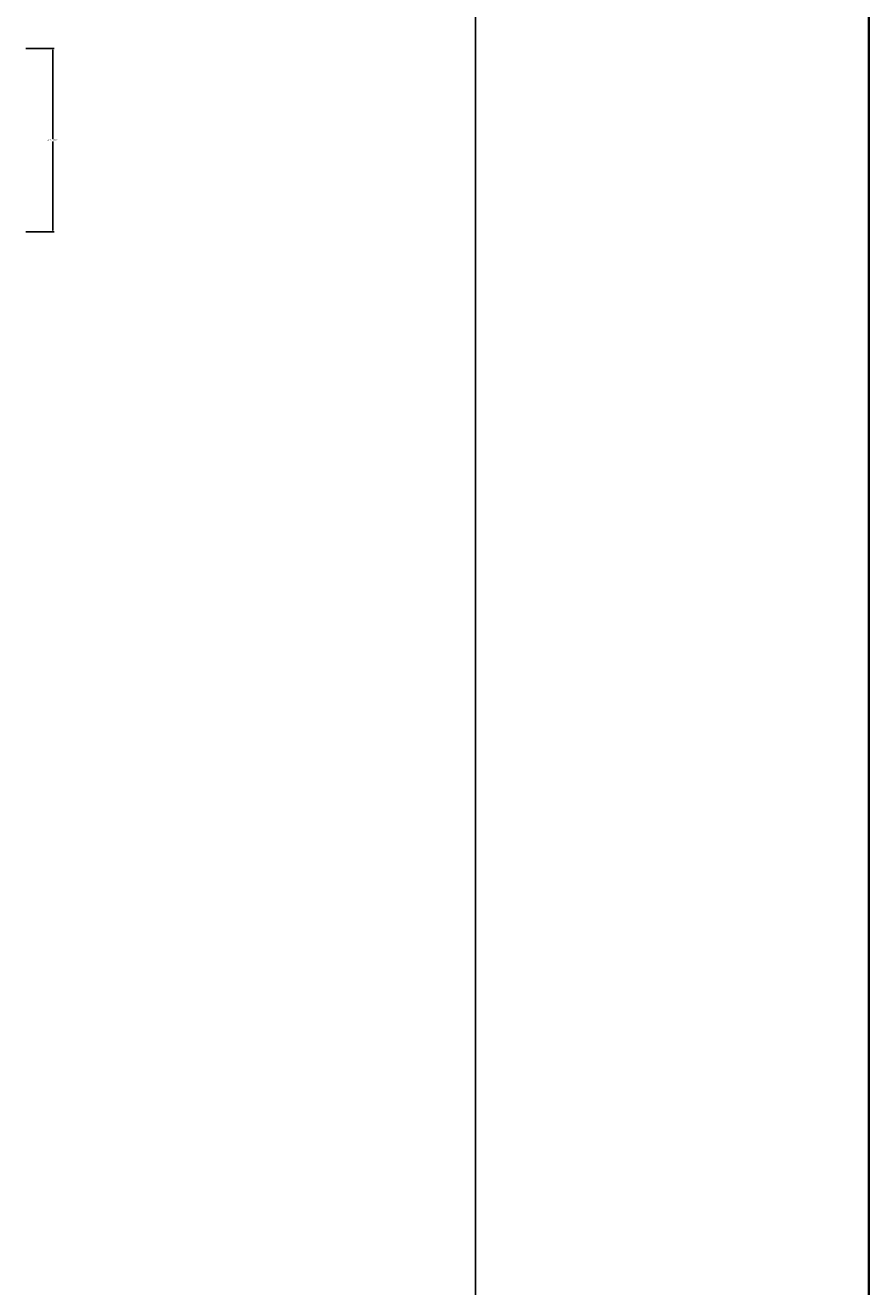
# Model space of a CAD drawing. Units: inches. Extents: x 1962 to 2771, y 1245 to 2660.
# Tile 19 of 114: x 2661 to 2771, y 1527 to 1692. Entities that reach past the tile are written whole.
import ezdxf

# ---------------------------------------------------------------- set-up
doc = ezdxf.new("R2010")
doc.units = ezdxf.units.IN
doc.layers.add('A-ANNO-DIMS', color=2, linetype='Continuous', lineweight=18)
doc.layers.add('A-ANNO-TTLB', color=7, linetype='Continuous', lineweight=35)
doc.styles.get("Standard").update_dxf_attribs({"font": 'arial.ttf'})
doc.dimstyles.get("Standard").update_dxf_attribs({"dimtxt": 0.18, "dimasz": 0.18, "dimexe": 0.18, "dimexo": 0.0625, "dimgap": 0.09, "dimtad": 0, "dimtih": 1, "dimtoh": 1, "dimdec": 4, "dimzin": 0, "dimdsep": 46, "dimtxsty": 'Standard', "dimcen": 0.09, "dimadec": 0, "dimazin": 0, "dimtfac": 1, "dimtdec": 4, "dimtofl": 0, "dimtmove": 0, "dimatfit": 3, "dimfxl": 1, "dimtolj": 1, "dimtzin": 0, "dimarcsym": 0})

# ---------------------------------------------------------------- blocks, each defined once
blk = doc.blocks.new('*D18')
at = {"layer": 'A-ANNO-DIMS', "color": 0, "lineweight": -2, "transparency": 16777216}
for p, q in [((2660.87, 1688.97), (2664.59, 1688.97)), ((2664.41, 1688.79), (2664.41, 1677.15)), ((2664.41, 1665.15), (2664.41, 1676.79)), ((2660.87, 1664.97), (2664.59, 1664.97))]:
    blk.add_line(p, q, dxfattribs=at)
at = {"layer": 'A-ANNO-DIMS', "color": 0, "transparency": 16777216}
for points in [[(2664.38, 1688.79), (2664.44, 1688.79), (2664.41, 1688.97)], [(2664.38, 1665.15), (2664.44, 1665.15), (2664.41, 1664.97)]]:
    blk.add_solid(points, dxfattribs=at)
at = {"layer": 'Defpoints', "color": 0, "transparency": 16777216}
for p in [(2660.81, 1688.97), (2664.41, 1688.97), (2660.81, 1664.97)]:
    blk.add_point(p, dxfattribs=at)
at = {"layer": 'A-ANNO-DIMS', "color": 0, "transparency": 16777216, "insert": (2664.41, 1676.97), "char_height": 0.18, "attachment_point": 5}
blk.add_mtext('\\A1;W1A 24 TYP.', dxfattribs=at)
blk = doc.blocks.new('*D42')
at = {"layer": 'A-ANNO-DIMS', "color": 0, "lineweight": -2, "transparency": 16777216}
for p, q in [((2660.87, 2524.34), (2719.94, 2524.34)), ((2719.76, 2524.16), (2719.76, 1979.28)), ((2719.76, 1434.02), (2719.76, 1978.91)), ((2660.87, 1433.84), (2719.94, 1433.84))]:
    blk.add_line(p, q, dxfattribs=at)
at = {"layer": 'A-ANNO-DIMS', "color": 0, "transparency": 16777216}
for points in [[(2719.73, 2524.16), (2719.79, 2524.16), (2719.76, 2524.34)], [(2719.73, 1434.02), (2719.79, 1434.02), (2719.76, 1433.84)]]:
    blk.add_solid(points, dxfattribs=at)
at = {"layer": 'Defpoints', "color": 0, "transparency": 16777216}
for p in [(2660.81, 2524.34), (2719.76, 2524.34), (2660.81, 1433.84)]:
    blk.add_point(p, dxfattribs=at)
at = {"layer": 'A-ANNO-DIMS', "color": 0, "transparency": 16777216, "insert": (2719.76, 1979.09), "char_height": 0.18, "attachment_point": 5}
blk.add_mtext('\\A1;1090.5', dxfattribs=at)

msp = doc.modelspace()

# ---------------------------------------------------------------- linework, layer by layer
at = {"layer": 'A-ANNO-TTLB'}
msp.add_lwpolyline([(1961.7365, 2660.2579), (2771.213, 2660.2579), (2771.213, 1244.5817), (1961.7365, 1244.5817)], close=True, dxfattribs=at)

# ---------------------------------------------------------------- dimensions: what is measured, and where the dimension line sits
at = {"layer": 'A-ANNO-DIMS'}
dim = msp.add_linear_dim(base=(2719.7574, 2524.3437), p1=(2660.8074, 1433.8437), p2=(2660.8074, 2524.3437), angle=90, dimstyle='Standard', override={"dimdec": 1, "dimlfac": 1, "dimrnd": 0, "dimzin": 0, "dimdsep": 46, "dimlunit": 2}, dxfattribs=at)
dim.commit()
dim.dimension.update_dxf_attribs({"geometry": '*D42', "text_midpoint": (2719.7574, 1979.0937)})
dim = msp.add_linear_dim(base=(2664.4074, 1688.9663), p1=(2660.8074, 1664.9663), p2=(2660.8074, 1688.9663), angle=90, text='W1A <> TYP.', dimstyle='Standard', override={"dimdec": 0, "dimlfac": 1, "dimrnd": 0, "dimzin": 0, "dimdsep": 46, "dimlunit": 2}, dxfattribs=at)
dim.commit()
dim.dimension.update_dxf_attribs({"geometry": '*D18', "text_midpoint": (2664.4074, 1676.9663)})

doc.saveas('drawing.dxf')
